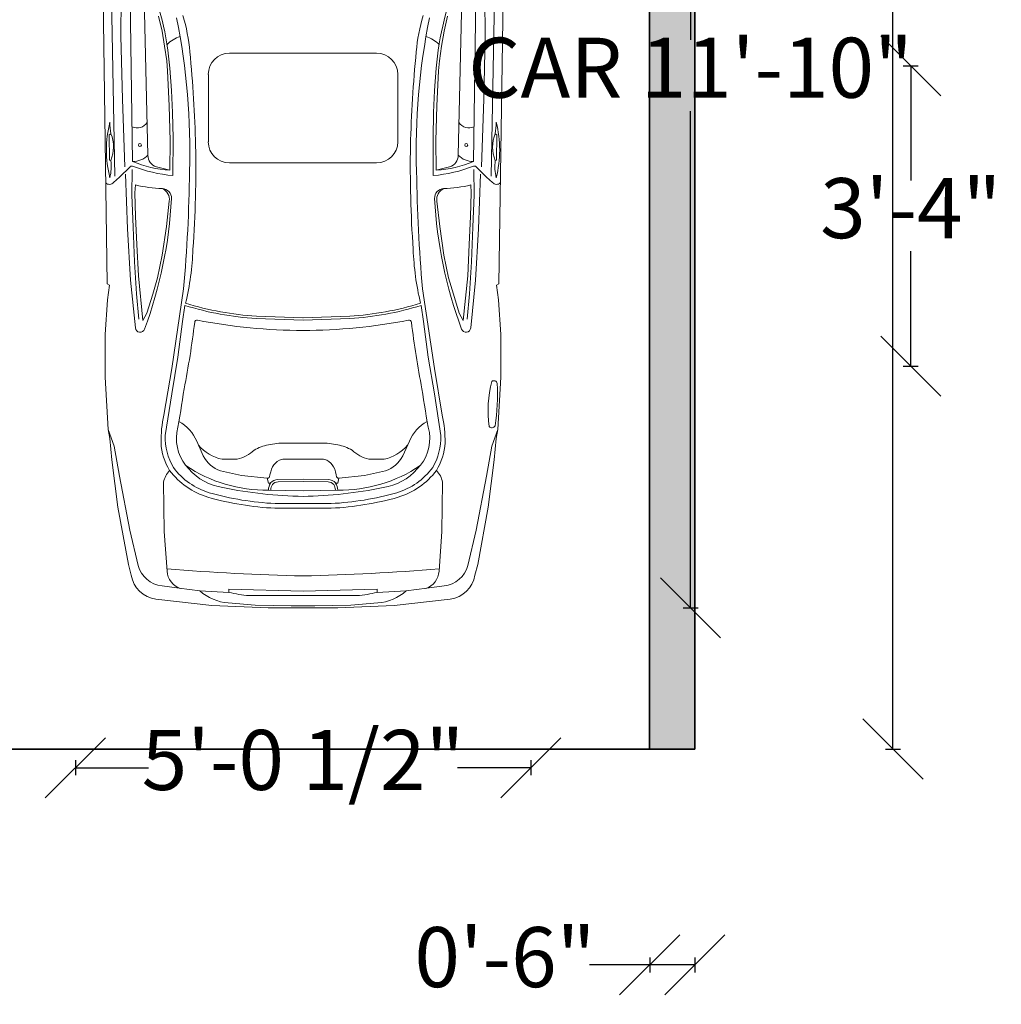
# Model space of a CAD drawing. Units: inches. Extents: x 2247 to 2713, y 588 to 1209.
# Tile 2 of 5: x 2574 to 2705, y 594 to 725. Entities that reach past the tile are written whole.
import ezdxf

# ---------------------------------------------------------------- set-up
doc = ezdxf.new("R2010")
doc.units = ezdxf.units.IN
for name, color, linetype, lineweight in [('0_Equip', 250, 'Continuous', 18), ('A-ANNO-DIMS', 2, 'Continuous', 18), ('A-WALL', 7, 'Continuous', 35), ('A-WALL-PATT', 4, 'Continuous', 13)]:
    doc.layers.add(name, color=color, linetype=linetype, lineweight=lineweight)
doc.styles.get("Standard").update_dxf_attribs({"font": 'arial.ttf'})
doc.dimstyles.new('ISO-25', dxfattribs={"dimtxt": 8, "dimasz": 8, "dimexe": 1, "dimexo": 1, "dimtad": 0, "dimtih": 1, "dimtoh": 1, "dimlunit": 3, "dimtxsty": 'Standard', "dimblk": 'OBLIQUE', "dimcen": 2.5, "dimadec": 0, "dimazin": 0, "dimtfac": 1, "dimtmove": 0, "dimatfit": 3, "dimfxl": 1, "dimfxlon": 1, "dimarcsym": 0})

# ---------------------------------------------------------------- blocks, each defined once
blk = doc.blocks.new('A$C4C7B54D1')
at = {"layer": '0_Equip', "ltscale": 0.1}
for p, q in [((-1.5337, 0.8406), (-1.5355, 0.484)), ((-1.4835, -0.0735), (-1.497, 0.863)), ((0.0322, -0.0735), (0.0457, 0.863)), ((0.0824, 0.8406), (0.0842, 0.484)), ((-1.6171, 0.8152), (-1.5964, -0.6171)), ((-1.5805, 0.8299), (-1.5623, -0.138)), ((-1.4352, 0.792), (-1.4152, -0.045)), ((-0.0162, 0.792), (-0.0361, -0.045)), ((0.1292, 0.8299), (0.111, -0.138)), ((0.1658, 0.8152), (0.145, -0.6171)), ((-1.368, 0.5729), (-1.3527, 0.5066)), ((-0.0834, 0.5729), (-0.0986, 0.5066)), ((-1.5355, 0.484), (-1.5292, 0.2045)), ((-1.3527, 0.5066), (-1.3411, 0.4394)), ((-0.0986, 0.5066), (-0.1102, 0.4394)), ((0.0842, 0.484), (0.0779, 0.2045)), ((-1.3411, 0.4394), (-1.3321, 0.3749)), ((-0.1102, 0.4394), (-0.1192, 0.3749)), ((-0.7257, 0.4085), (-1.0528, 0.4085)), ((-0.7257, 0.4085), (-0.3986, 0.4085)), ((-1.3321, 0.3749), (-1.3286, 0.3301)), ((-0.1192, 0.3749), (-0.1228, 0.3301)), ((-1.3286, 0.3301), (-1.3204, 0.1751)), ((-1.3178, 0.3418), (-1.31, 0.2426)), ((-1.1468, 0.3145), (-1.1468, 0.0145)), ((-0.3045, 0.3145), (-0.3045, 0.0145)), ((-0.1335, 0.3418), (-0.1413, 0.2426)), ((-0.1228, 0.3301), (-0.1309, 0.1751)), ((-1.31, 0.2426), (-1.306, 0.1454)), ((-0.1413, 0.2426), (-0.1454, 0.1454)), ((-1.5292, 0.2045), (-1.5185, -0.0974)), ((0.0779, 0.2045), (0.0672, -0.0974)), ((-1.3204, 0.1751), (-1.3164, 0.0193)), ((-1.306, 0.1454), (-1.3036, 0.0305)), ((-0.1454, 0.1454), (-0.1478, 0.0305)), ((-0.1309, 0.1751), (-0.1349, 0.0193)), ((-1.5798, 0.0505), (-1.5879, 0.0456)), ((-1.5879, 0.0456), (-1.5863, -0.0676)), ((0.1285, 0.0505), (0.1365, 0.0456)), ((0.1365, 0.0456), (0.1349, -0.0676)), ((-1.3164, 0.0193), (-1.3178, -0.1112)), ((-1.3036, 0.0305), (-1.3044, -0.1358)), ((-0.1478, 0.0305), (-0.147, -0.1358)), ((-0.1349, 0.0193), (-0.1335, -0.1112)), ((-1.5863, -0.0676), (-1.5806, -0.0692)), ((-0.7257, -0.0796), (-1.0528, -0.0796)), ((-0.7257, -0.0796), (-0.3986, -0.0796)), ((0.1349, -0.0676), (0.1293, -0.0692)), ((-1.4948, -0.0965), (-1.5413, -0.143)), ((-1.5147, -0.1299), (-1.5058, -0.3725)), ((-1.4857, -0.1082), (-1.4866, -0.2223)), ((-1.3774, -0.0972), (-1.3178, -0.1112)), ((-0.0739, -0.0972), (-0.1335, -0.1112)), ((0.0344, -0.1082), (0.0352, -0.2223)), ((0.0435, -0.0965), (0.0899, -0.143)), ((0.0633, -0.1299), (0.0545, -0.3725)), ((-1.5413, -0.143), (-1.5686, -0.1663)), ((0.0899, -0.143), (0.1172, -0.1663)), ((-1.4713, -0.1773), (-1.4737, -0.2127)), ((-1.4737, -0.2127), (-1.4705, -0.3187)), ((0.0224, -0.2127), (0.0192, -0.3187)), ((0.02, -0.1773), (0.0224, -0.2127)), ((-1.4866, -0.2223), (-1.4809, -0.3653)), ((-1.3211, -0.2496), (-1.3332, -0.3629)), ((-0.1302, -0.2496), (-0.1182, -0.3629)), ((0.0352, -0.2223), (0.0296, -0.3653)), ((-1.4705, -0.3187), (-1.4649, -0.4424)), ((0.0192, -0.3187), (0.0135, -0.4424)), ((-1.5058, -0.3725), (-1.4922, -0.6007)), ((-1.4809, -0.3653), (-1.4745, -0.5203)), ((-1.3332, -0.3629), (-1.3516, -0.4906)), ((-0.1182, -0.3629), (-0.0997, -0.4906)), ((0.0296, -0.3653), (0.0232, -0.5203)), ((0.0545, -0.3725), (0.0408, -0.6007)), ((-1.4649, -0.4424), (-1.4576, -0.5822)), ((0.0135, -0.4424), (0.0063, -0.5822)), ((-1.4745, -0.5203), (-1.4665, -0.6617)), ((-1.3516, -0.4906), (-1.3725, -0.5902)), ((-0.0997, -0.4906), (-0.0788, -0.5902)), ((0.0232, -0.5203), (0.0151, -0.6617)), ((-1.4922, -0.6007), (-1.4712, -0.814)), ((-1.4576, -0.5822), (-1.4384, -0.7806)), ((-1.3725, -0.5902), (-1.3942, -0.6641)), ((-0.0788, -0.5902), (-0.0571, -0.6641)), ((0.0063, -0.5822), (-0.013, -0.7806)), ((0.0408, -0.6007), (0.0198, -0.814)), ((-1.5964, -0.6171), (-1.5863, -0.6228)), ((-1.5863, -0.6228), (-1.5949, -0.6885)), ((-1.3094, -0.9936), (-1.2569, -0.6398)), ((-0.1419, -0.9936), (-0.1944, -0.6398)), ((0.145, -0.6171), (0.1349, -0.6228)), ((0.1349, -0.6228), (0.1436, -0.6885)), ((-1.5949, -0.6885), (-1.605, -0.843)), ((-1.4665, -0.6617), (-1.4552, -0.7742)), ((-1.3942, -0.6641), (-1.4199, -0.7485)), ((-0.0571, -0.6641), (-0.0314, -0.7485)), ((0.0151, -0.6617), (0.0039, -0.7742)), ((0.1436, -0.6885), (0.1537, -0.843)), ((-1.2616, -0.7846), (-1.2511, -0.7134)), ((-0.1898, -0.7846), (-0.2003, -0.7134)), ((-1.4199, -0.7485), (-1.4384, -0.7806)), ((-1.2826, -0.9445), (-1.2616, -0.7846)), ((-0.9336, -0.7717), (-0.7257, -0.7787)), ((-0.9331, -0.7613), (-0.7253, -0.7683)), ((-0.5182, -0.7613), (-0.726, -0.7683)), ((-0.5177, -0.7717), (-0.7257, -0.7787)), ((-0.1688, -0.9445), (-0.1898, -0.7846)), ((-0.0314, -0.7485), (-0.013, -0.7806)), ((-1.605, -0.843), (-1.605, -1.0322)), ((0.1537, -0.843), (0.1537, -1.0322)), ((-1.3094, -1.1068), (-1.2826, -0.9445)), ((-0.1419, -1.1068), (-0.1688, -0.9445)), ((-1.3444, -1.2014), (-1.3094, -0.9936)), ((-0.1069, -1.2014), (-0.1419, -0.9936)), ((-1.605, -1.0322), (-1.592, -1.2661)), ((0.1537, -1.0322), (0.1407, -1.2661)), ((-1.3386, -1.2925), (-1.3094, -1.1068)), ((-0.1127, -1.2925), (-0.1419, -1.1068)), ((-1.565, -1.3405), (-1.592, -1.2661)), ((-1.592, -1.2661), (-1.5848, -1.3051)), ((0.1137, -1.3405), (0.1407, -1.2661)), ((0.1407, -1.2661), (0.1335, -1.3051)), ((-1.5848, -1.3051), (-1.5762, -1.4004)), ((0.1335, -1.3051), (0.1248, -1.4004)), ((-1.5417, -1.4736), (-1.565, -1.3405)), ((-1.1985, -1.3182), (-1.1694, -1.3835)), ((-0.88, -1.3337), (-0.8328, -1.3271)), ((-0.8328, -1.3271), (-0.7257, -1.3271)), ((-0.6185, -1.3271), (-0.7257, -1.3271)), ((-0.5713, -1.3337), (-0.6185, -1.3271)), ((-0.2528, -1.3182), (-0.282, -1.3835)), ((0.0904, -1.4736), (0.1137, -1.3405)), ((-1.5762, -1.4004), (-1.5486, -1.6107)), ((-1.0858, -1.3979), (-1.0181, -1.3979)), ((-0.8163, -1.3979), (-0.8309, -1.402)), ((-0.7257, -1.3974), (-0.8163, -1.3979)), ((-0.7257, -1.3974), (-0.635, -1.3979)), ((-0.635, -1.3979), (-0.6204, -1.402)), ((-0.3655, -1.3979), (-0.4333, -1.3979)), ((0.1248, -1.4004), (0.0973, -1.6107)), ((-0.8664, -1.4423), (-0.8696, -1.4545)), ((-0.861, -1.4312), (-0.8664, -1.4423)), ((-0.8558, -1.4236), (-0.861, -1.4312)), ((-0.8488, -1.4158), (-0.8558, -1.4236)), ((-0.8409, -1.4088), (-0.8488, -1.4158)), ((-0.8309, -1.402), (-0.8409, -1.4088)), ((-0.6204, -1.402), (-0.6104, -1.4088)), ((-0.6104, -1.4088), (-0.6025, -1.4158)), ((-0.6025, -1.4158), (-0.5955, -1.4236)), ((-0.5955, -1.4236), (-0.5904, -1.4312)), ((-0.5904, -1.4312), (-0.585, -1.4423)), ((-0.585, -1.4423), (-0.5817, -1.4545)), ((-1.4962, -1.7129), (-1.5417, -1.4736)), ((-1.0923, -1.4501), (-0.9989, -1.4699)), ((-0.9989, -1.4699), (-0.8846, -1.4828)), ((-0.8807, -1.4821), (-0.8846, -1.4828)), ((-0.8846, -1.4828), (-0.8799, -1.5038)), ((-0.8769, -1.4791), (-0.8807, -1.4821)), ((-0.8745, -1.477), (-0.8769, -1.4791)), ((-0.8731, -1.467), (-0.8745, -1.477)), ((-0.8696, -1.4545), (-0.8731, -1.467)), ((-0.7257, -1.4865), (-0.8374, -1.4884)), ((-0.7257, -1.4865), (-0.6139, -1.4884)), ((-0.5817, -1.4545), (-0.5782, -1.467)), ((-0.5782, -1.467), (-0.5768, -1.477)), ((-0.5768, -1.477), (-0.5744, -1.4791)), ((-0.5744, -1.4791), (-0.5706, -1.4821)), ((-0.5668, -1.4828), (-0.5714, -1.5038)), ((-0.5706, -1.4821), (-0.5668, -1.4828)), ((-0.4524, -1.4699), (-0.5668, -1.4828)), ((-0.359, -1.4501), (-0.4524, -1.4699)), ((0.0448, -1.7129), (0.0904, -1.4736)), ((-1.3456, -1.5004), (-1.3433, -1.7188)), ((-0.8799, -1.5038), (-0.8706, -1.5038)), ((-0.7257, -1.4969), (-0.837, -1.4988)), ((-0.7257, -1.4969), (-0.6143, -1.4988)), ((-0.5714, -1.5038), (-0.5808, -1.5038)), ((-0.1057, -1.5004), (-0.1081, -1.7188)), ((-0.8799, -1.5352), (-0.7257, -1.5393)), ((-0.5714, -1.5352), (-0.7257, -1.5393)), ((-1.5486, -1.6107), (-1.5024, -1.8663)), ((-0.8507, -1.616), (-0.7257, -1.616)), ((-0.8502, -1.5951), (-0.7257, -1.5951)), ((-0.6011, -1.5951), (-0.7257, -1.5951)), ((-0.6006, -1.616), (-0.7257, -1.616)), ((0.0973, -1.6107), (0.0511, -1.8663)), ((-1.4584, -1.8701), (-1.4962, -1.7129)), ((-1.3433, -1.7188), (-1.3304, -1.8962)), ((-0.1081, -1.7188), (-0.1209, -1.8962)), ((0.0071, -1.8701), (0.0448, -1.7129)), ((-1.5024, -1.8663), (-1.4894, -1.914)), ((0.0511, -1.8663), (0.0381, -1.914)), ((-1.2767, -1.9721), (-1.3526, -1.9616)), ((-0.1746, -1.9721), (-0.0987, -1.9616)), ((-1.1845, -1.9838), (-1.2767, -1.9721)), ((-1.055, -1.9908), (-1.1845, -1.9838)), ((-1.055, -1.9768), (-1.055, -1.9908)), ((-0.7257, -1.985), (-1.055, -1.9768)), ((-0.9663, -2.0048), (-0.7257, -2.0048)), ((-0.7257, -1.985), (-0.3964, -1.9768)), ((-0.4851, -2.0048), (-0.7257, -2.0048)), ((-0.3964, -1.9768), (-0.3964, -1.9908)), ((-0.3964, -1.9908), (-0.2668, -1.9838)), ((-0.2668, -1.9838), (-0.1746, -1.9721)), ((-1.3797, -2.0208), (-1.1314, -2.0483)), ((-1.1314, -2.0483), (-0.8803, -2.0598)), ((-1.0585, -2.0375), (-0.9383, -2.0469)), ((-0.9383, -2.0469), (-0.7784, -2.0504)), ((-0.7784, -2.0504), (-0.7257, -2.0504)), ((-0.673, -2.0504), (-0.7257, -2.0504)), ((-0.5131, -2.0469), (-0.673, -2.0504)), ((-0.3199, -2.0483), (-0.5711, -2.0598)), ((-0.3929, -2.0375), (-0.5131, -2.0469)), ((-0.0716, -2.0208), (-0.3199, -2.0483)), ((-0.8803, -2.0598), (-0.7257, -2.0598)), ((-0.5711, -2.0598), (-0.7257, -2.0598))]:
    blk.add_line(p, q, dxfattribs=at)
for centre in [(-1.4513, 0), (0, 0)]:
    blk.add_circle(centre, 0.00662, dxfattribs=at)
for centre, radius, start, end in [((-6.6059, -0.8606), 5.4408, 15.0904, 20.5451), ((5.1546, -0.8606), 5.4408, 159.4549, 164.9096), ((-2.0025, 0.3511), 0.7759, 4.7259, 16.8296), ((0.5512, 0.3511), 0.7759, 163.1704, 175.2741), ((-2.6334, 0.2371), 1.3197, 4.5498, 13.9797), ((-4.2099, -0.0242), 2.9809, 358.1905, 11.4064), ((2.7585, -0.0242), 2.9809, 168.5936, 181.8095), ((1.1821, 0.2371), 1.3197, 166.0203, 175.4502), ((-1.2324, 0.3484), 0.1397, 106.6168, 134.6647), ((-0.2189, 0.3484), 0.1397, 45.3353, 73.3832), ((-6.5594, -0.126), 5.3575, 1.3159, 5.7952), ((-1.0528, 0.3145), 0.0941, 90, 180), ((-0.3986, 0.3145), 0.0941, 0, 90), ((5.1081, -0.126), 5.3575, 174.2048, 178.6841), ((-1.0944, -0.0222), 0.5055, 165.8807, 194.1193), ((-1.3066, 0.102), 0.2781, 180.1936, 190.6834), ((-1.4634, 0.1296), 0.0534, 245.2796, 326.9469), ((0.0121, 0.1296), 0.0534, 213.0531, 294.7204), ((-0.1448, 0.102), 0.2781, 349.3166, 359.8064), ((-0.3569, -0.0222), 0.5055, 345.8807, 14.1193), ((-1.7275, -0.0084), 0.159, 337.4976, 21.7335), ((0.2762, -0.0084), 0.159, 158.2665, 202.5024), ((-1.0528, 0.0145), 0.0941, 180, 270), ((-0.3986, 0.0145), 0.0941, 270, 0), ((-6.573, -0.0941), 5.3705, 356.0501, 0.9723), ((5.1217, -0.0941), 5.3705, 179.0277, 183.9499), ((-1.7817, -0.0969), 0.2029, 346.1346, 7.8419), ((-1.4831, 0.0214), 0.095, 269.7172, 315.6185), ((-1.2968, 0.3651), 0.4767, 246.9385, 267.4714), ((-1.3634, -0.0473), 0.0519, 177.4537, 254.2676), ((-0.1545, 0.3651), 0.4767, 272.5286, 293.0615), ((-0.0879, -0.0473), 0.0519, 285.7324, 2.5463), ((0.0317, 0.0214), 0.095, 224.3815, 270.2828), ((0.3303, -0.0969), 0.2029, 172.1581, 193.8654), ((-1.4874, -0.1039), 0.0105, 68.8598, 135.0096), ((-1.2476, 0.5164), 0.6547, 248.8598, 265.0222), ((-8.0298, -0.0355), 6.7998, 354.90123, 359.30214), ((6.5785, -0.0355), 6.7998, 180.69786, 185.09877), ((-0.2038, 0.5164), 0.6547, 274.9778, 291.1402), ((0.0361, -0.1039), 0.0105, 44.9904, 111.1402), ((-1.5869, -0.1514), 0.0236, 227.2909, 320.7388), ((0.1355, -0.1514), 0.0236, 219.2612, 312.7091), ((-1.3362, 0.3542), 0.5484, 255.7347, 268.4072), ((-1.3699, -0.2402), 0.0497, 349.0381, 68.1064), ((-1.3526, -0.2358), 0.0418, 357.143, 88.4072), ((-0.0988, -0.2358), 0.0418, 91.5928, 182.857), ((-0.0814, -0.2402), 0.0497, 111.8936, 190.9619), ((-0.1152, 0.3542), 0.5484, 271.5928, 284.2653), ((-3.2483, -0.1412), 1.9399, 339.54, 357.143), ((1.797, -0.1412), 1.9399, 182.857, 200.46), ((-2.454, -0.4173), 1.2396, 346.6558, 357.8401), ((1.0027, -0.4173), 1.2396, 182.1599, 193.3442), ((-0.8588, 0.5276), 1.3014, 252.4566, 266.7043), ((-0.8588, 0.5276), 1.291, 252.4566, 266.6988), ((-0.5926, 0.5276), 1.291, 273.3012, 287.5434), ((-0.5926, 0.5276), 1.3014, 273.2957, 287.5434), ((-1.1971, -0.7899), 0.0105, 79.1189, 173.1671), ((-0.7142, 1.7227), 2.5481, 259.1189, 269.7413), ((-0.7372, 1.7227), 2.5481, 270.2587, 280.8811), ((-0.2542, -0.7899), 0.0105, 6.8329, 100.8811), ((-1.4504, -0.812), 0.0209, 185.6259, 339.54), ((-5.088, -0.3237), 3.9082, 348.7726, 353.1671), ((3.6366, -0.3237), 3.9082, 186.8329, 191.2274), ((-0.001, -0.812), 0.0209, 200.46, 354.3741), ((0.1224, -1.0639), 0.0155, 11.61, 127.0083), ((-4.7286, -0.6026), 3.5073, 348.8701, 352.1003), ((3.2772, -0.6026), 3.5073, 187.8997, 191.1299), ((0.625, -1.1812), 0.5281, 165.7822, 187.813), ((-0.7003, -1.1122), 0.8395, 350.5693, 3.5107), ((-0.8187, -1.3185), 0.5386, 167.4447, 180.7102), ((-0.6326, -1.3185), 0.5386, 359.2898, 12.5553), ((-1.3591, -1.3822), 0.1728, 21.7432, 61.9432), ((-0.0922, -1.3822), 0.1728, 118.0568, 158.2568), ((0.1138, -1.243), 0.0156, 219.7819, 334.4738), ((-1.0611, -1.2979), 0.2775, 178.8811, 209.7062), ((-1.0952, -1.3051), 0.1937, 172.4314, 224.4267), ((-0.3561, -1.3051), 0.1937, 315.5733, 7.5686), ((-0.3902, -1.2979), 0.2775, 330.2938, 1.1189), ((-1.0944, -1.3104), 0.2633, 183.2136, 211.504), ((-1.0482, -1.2146), 0.1871, 220.4031, 258.3959), ((-1.0495, -1.2507), 0.1505, 282.0448, 314.7653), ((-0.8301, -1.5634), 0.235, 102.268, 118.8572), ((-0.6213, -1.5634), 0.235, 61.1428, 77.732), ((-0.4019, -1.2507), 0.1505, 225.2347, 257.9552), ((-0.4032, -1.2146), 0.1871, 281.6041, 319.5969), ((-0.3569, -1.3104), 0.2633, 328.496, 356.7864), ((-1.0421, -1.3141), 0.145, 208.6187, 249.7318), ((-0.4092, -1.3141), 0.145, 290.2682, 331.3813), ((-1.052, -1.2472), 0.313, 216.9484, 253.2054), ((-0.8912, -0.9022), 0.6331, 235.8724, 271.0227), ((-1.0459, -1.2776), 0.2487, 221.0065, 261.6946), ((-0.5601, -0.9022), 0.6331, 268.9773, 304.1276), ((-0.4054, -1.2776), 0.2487, 278.3054, 318.9935), ((-0.3993, -1.2472), 0.313, 286.7946, 323.0516), ((-1.2501, -1.516), 0.0967, 135.2951, 170.7274), ((-1.052, -1.2472), 0.3339, 216.9484, 253.2314), ((-0.8344, -1.538), 0.0498, 93.4455, 136.5439), ((-0.6169, -1.538), 0.0498, 43.4561, 86.5545), ((-0.3993, -1.2472), 0.3339, 286.7686, 323.0516), ((-0.2012, -1.516), 0.0967, 9.2726, 44.7049), ((-0.7003, 0.2815), 1.8451, 258.0669, 269.2129), ((-0.8066, -1.54), 0.0735, 150.5285, 176.2825), ((-0.8066, -1.54), 0.063, 151.7195, 175.9212), ((-0.8344, -1.538), 0.0393, 93.7549, 134.7116), ((-0.751, 0.2815), 1.8451, 270.7871, 281.9331), ((-0.6169, -1.538), 0.0393, 45.2884, 86.2451), ((-0.6447, -1.54), 0.063, 4.0788, 28.2805), ((-0.6447, -1.54), 0.0735, 3.7175, 29.4715), ((-0.7884, -0.3101), 1.3074, 254.0198, 267.2681), ((-0.7884, -0.3101), 1.2865, 254.0263, 267.246), ((-0.6629, -0.3101), 1.2865, 272.754, 285.9737), ((-0.6629, -0.3101), 1.3074, 272.7319, 285.9802), ((-1.3393, -1.8393), 0.123, 194.4986, 263.7836), ((-0.1121, -1.8393), 0.123, 276.2164, 345.5014), ((-1.3628, -1.8937), 0.1282, 189.093, 262.4153), ((-0.5134, 7.9307), 9.8503, 265.23745, 268.76503), ((-1.2452, -1.8915), 0.0853, 183.2055, 252.6405), ((-0.938, 7.9307), 9.8503, 271.23497, 274.76255), ((-0.2061, -1.8915), 0.0853, 287.3595, 356.7945), ((-0.0885, -1.8937), 0.1282, 277.5847, 350.907), ((-1.0413, -1.8225), 0.2157, 228.406, 265.4391), ((-0.896, -1.272), 0.7362, 257.5275, 264.5209), ((-0.5554, -1.272), 0.7362, 275.4791, 282.4725), ((-0.41, -1.8225), 0.2157, 274.5609, 311.594)]:
    blk.add_arc(centre, radius, start, end, dxfattribs=at)
blk = doc.blocks.new('_Oblique')
at = {"color": 0, "linetype": 'ByBlock', "lineweight": -2}
blk.add_line((-0.5, -0.5), (0.5, 0.5), dxfattribs=at)
blk = doc.blocks.new('*D12')
at = {"layer": 'A-ANNO-DIMS', "color": 0, "lineweight": -2, "transparency": 16777216}
for p, q in [((2689.46, 1168.28), (2691.46, 1168.28)), ((2690.46, 1168.28), (2690.46, 902.97)), ((2690.46, 628.28), (2690.46, 893.59)), ((2689.46, 628.28), (2691.46, 628.28))]:
    blk.add_line(p, q, dxfattribs=at)
at = {"layer": 'Defpoints', "color": 0, "transparency": 16777216}
for p in [(2664.08, 1168.28), (2664.08, 628.28), (2690.46, 628.28)]:
    blk.add_point(p, dxfattribs=at)
at = {"layer": 'A-ANNO-DIMS', "color": 0, "lineweight": -2, "transparency": 16777216, "xscale": 8, "yscale": 8, "zscale": 8}
for p, rotation in [((2690.46, 1168.28), 90), ((2690.46, 628.28), 270)]:
    blk.add_blockref('_Oblique', p, dxfattribs=dict(at, rotation=rotation))
at = {"layer": 'A-ANNO-DIMS', "color": 0, "transparency": 16777216, "insert": (2690.46, 898.28), "char_height": 8, "attachment_point": 5}
blk.add_mtext("45'", dxfattribs=at)
blk = doc.blocks.new('*D23')
at = {"layer": 'A-ANNO-DIMS', "color": 0, "lineweight": -2, "transparency": 16777216}
for p, q in [((2662.52, 788.89), (2664.52, 788.89)), ((2663.52, 788.89), (2663.52, 722.74)), ((2663.52, 647.07), (2663.52, 713.22)), ((2662.52, 647.07), (2664.52, 647.07))]:
    blk.add_line(p, q, dxfattribs=at)
at = {"layer": 'Defpoints', "color": 0, "transparency": 16777216}
for p in [(2642.25, 788.89), (2663.52, 788.89), (2642.25, 647.07)]:
    blk.add_point(p, dxfattribs=at)
at = {"layer": 'A-ANNO-DIMS', "color": 0, "lineweight": -2, "transparency": 16777216, "xscale": 8, "yscale": 8, "zscale": 8}
for p, rotation in [((2663.52, 788.89), 90), ((2663.52, 647.07), 270)]:
    blk.add_blockref('_Oblique', p, dxfattribs=dict(at, rotation=rotation))
at = {"layer": 'A-ANNO-DIMS', "color": 0, "transparency": 16777216, "insert": (2663.52, 717.98), "char_height": 8, "attachment_point": 5}
blk.add_mtext('CAR 11\'-10"', dxfattribs=at)
blk = doc.blocks.new('*D24')
at = {"layer": 'A-ANNO-DIMS', "color": 0, "lineweight": -2, "transparency": 16777216}
for p, q in [((2581.64, 626.79), (2581.64, 624.79)), ((2581.64, 625.79), (2591.36, 625.79)), ((2642.25, 625.79), (2632.52, 625.79)), ((2642.25, 626.79), (2642.25, 624.79))]:
    blk.add_line(p, q, dxfattribs=at)
at = {"layer": 'Defpoints', "color": 0, "transparency": 16777216}
for p in [(2581.64, 647.07), (2642.25, 647.07), (2642.25, 625.79)]:
    blk.add_point(p, dxfattribs=at)
at = {"layer": 'A-ANNO-DIMS', "color": 0, "lineweight": -2, "transparency": 16777216, "xscale": 8, "yscale": 8, "zscale": 8, "rotation": 180}
blk.add_blockref('_Oblique', (2581.64, 625.79), dxfattribs=at)
at = {"layer": 'A-ANNO-DIMS', "color": 0, "lineweight": -2, "transparency": 16777216, "xscale": 8, "yscale": 8, "zscale": 8}
blk.add_blockref('_Oblique', (2642.25, 625.79), dxfattribs=at)
at = {"layer": 'A-ANNO-DIMS', "color": 0, "transparency": 16777216, "insert": (2611.94, 625.79), "char_height": 8, "attachment_point": 5}
blk.add_mtext('5\'-0 1/2"', dxfattribs=at)
blk = doc.blocks.new('*D25')
at = {"layer": 'A-ANNO-DIMS', "color": 0, "lineweight": -2, "transparency": 16777216}
for p, q in [((2691.83, 719.28), (2693.83, 719.28)), ((2692.83, 719.28), (2692.83, 703.99)), ((2692.83, 679.28), (2692.83, 694.57)), ((2691.83, 679.28), (2693.83, 679.28))]:
    blk.add_line(p, q, dxfattribs=at)
at = {"layer": 'Defpoints', "color": 0, "transparency": 16777216}
for p in [(2520.08, 719.28), (2692.83, 719.28), (2520.08, 679.28)]:
    blk.add_point(p, dxfattribs=at)
at = {"layer": 'A-ANNO-DIMS', "color": 0, "lineweight": -2, "transparency": 16777216, "xscale": 8, "yscale": 8, "zscale": 8}
for p, rotation in [((2692.83, 719.28), 90), ((2692.83, 679.28), 270)]:
    blk.add_blockref('_Oblique', p, dxfattribs=dict(at, rotation=rotation))
at = {"layer": 'A-ANNO-DIMS', "color": 0, "transparency": 16777216, "insert": (2692.83, 699.28), "char_height": 8, "attachment_point": 5}
blk.add_mtext('3\'-4"', dxfattribs=at)
blk = doc.blocks.new('*D28')
at = {"layer": 'A-ANNO-DIMS', "color": 0, "lineweight": -2, "transparency": 16777216}
for p, q in [((2658.08, 599.53), (2650.08, 599.53)), ((2658.08, 600.53), (2658.08, 598.53)), ((2664.08, 599.53), (2658.08, 599.53)), ((2664.08, 600.53), (2664.08, 598.53))]:
    blk.add_line(p, q, dxfattribs=at)
at = {"layer": 'Defpoints', "color": 0, "transparency": 16777216}
for p in [(2658.08, 628.28), (2664.08, 628.28), (2658.08, 599.53)]:
    blk.add_point(p, dxfattribs=at)
at = {"layer": 'A-ANNO-DIMS', "color": 0, "lineweight": -2, "transparency": 16777216, "xscale": 8, "yscale": 8, "zscale": 8, "rotation": 180}
blk.add_blockref('_Oblique', (2658.08, 599.53), dxfattribs=at)
at = {"layer": 'A-ANNO-DIMS', "color": 0, "lineweight": -2, "transparency": 16777216, "xscale": 8, "yscale": 8, "zscale": 8}
blk.add_blockref('_Oblique', (2664.08, 599.53), dxfattribs=at)
at = {"layer": 'A-ANNO-DIMS', "color": 0, "transparency": 16777216, "insert": (2638.82, 599.53), "char_height": 8, "attachment_point": 5}
blk.add_mtext('0\'-6"', dxfattribs=at)

msp = doc.modelspace()

# ---------------------------------------------------------------- hatches: boundary and pattern name
at = {"layer": 'A-WALL-PATT'}
h = msp.add_hatch(color=256, dxfattribs=at)
h.dxf.hatch_style = 1
h.paths.add_polyline_path([(2604.041, 1168.28), (2423.716, 1168.28), (2423.716, 1162.28), (2442.076, 1162.28), (2442.076, 1114.28), (2439.021, 1114.28), (2439.021, 1108.28), (2456.056, 1108.28), (2456.056, 1114.28), (2448.076, 1114.28), (2448.076, 1162.28), (2580.076, 1162.28), (2580.076, 1114.28), (2560.507, 1114.28), (2560.507, 1108.28), (2619.195, 1108.28), (2619.195, 1114.28), (2586.076, 1114.28), (2586.076, 1162.28), (2604.041, 1162.28)])
h.paths.add_polyline_path([(2380.833, 1168.28), (2364.076, 1168.28), (2364.076, 1094.128), (2370.076, 1094.128), (2370.076, 1108.28), (2407.021, 1108.28), (2407.021, 1114.28), (2370.076, 1114.28), (2370.076, 1162.28), (2380.833, 1162.28)])
h.paths.add_polyline_path([(2664.076, 1168.28), (2639.393, 1168.28), (2639.393, 1162.28), (2658.076, 1162.28), (2658.076, 1114.28), (2651.195, 1114.28), (2651.195, 1108.28), (2658.076, 1108.28), (2658.076, 1094.128), (2664.076, 1094.128)])
h.paths.add_polyline_path([(2524.66, 1114.28), (2487.371, 1114.28), (2487.371, 1108.28), (2511.076, 1108.28), (2511.076, 940.28), (2508.076, 940.28), (2508.076, 934.28), (2520.076, 934.28), (2520.076, 940.28), (2517.076, 940.28), (2517.076, 1108.28), (2524.66, 1108.28)])
h.paths.add_polyline_path([(2370.076, 1054.172), (2364.076, 1054.172), (2364.076, 990.686), (2370.076, 990.686)])
h.paths.add_polyline_path([(2370.076, 934.28), (2472.076, 934.28), (2472.076, 940.28), (2370.076, 940.28), (2370.076, 950.99), (2364.076, 950.99), (2364.076, 902.687), (2370.076, 902.687)])
h.paths.add_polyline_path([(2664.076, 950.99), (2658.076, 950.99), (2658.076, 940.28), (2556.076, 940.28), (2556.076, 934.28), (2658.076, 934.28), (2658.076, 913.24), (2664.076, 913.24)])
h.paths.add_polyline_path([(2664.076, 1054.172), (2658.076, 1054.172), (2658.076, 990.686), (2664.076, 990.686)])
h.paths.add_polyline_path([(2664.076, 861.585), (2658.076, 861.585), (2658.076, 814.28), (2626.201, 814.28), (2626.201, 808.28), (2658.076, 808.28), (2658.076, 628.28), (2664.076, 628.28)])
h.paths.add_polyline_path([(2562.076, 871.28), (2556.076, 871.28), (2556.076, 808.28), (2584.934, 808.28), (2584.934, 814.28), (2562.076, 814.28)])
h.paths.add_polyline_path([(2475.722, 808.28), (2370.076, 808.28), (2370.076, 776.746), (2364.076, 776.746), (2364.076, 846.663), (2370.076, 846.663), (2370.076, 814.28), (2475.722, 814.28)])
h.paths.add_polyline_path([(2370.076, 709.673), (2364.076, 709.673), (2364.076, 628.28), (2520.076, 628.28), (2520.076, 634.28), (2370.076, 634.28)])
h.paths.add_polyline_path([(2410.479, 679.28), (2370.076, 679.28), (2370.076, 673.28), (2410.479, 673.28)], flags=17)
h.paths.add_polyline_path([(2520.076, 679.28), (2514.076, 679.28), (2474.076, 679.28), (2457.582, 679.28), (2457.582, 673.28), (2520.076, 673.28)], flags=17)
h.paths.add_polyline_path([(2520.076, 814.28), (2511.722, 814.28), (2511.722, 808.28), (2514.076, 808.28), (2514.076, 719.28), (2520.076, 719.28)])

# ---------------------------------------------------------------- linework, layer by layer
at = {"layer": 'A-WALL'}
for p, q in [((2664.076, 628.28), (2664.076, 1168.28)), ((2658.076, 628.28), (2658.076, 808.28)), ((2364.076, 628.28), (2664.076, 628.28))]:
    msp.add_line(p, q, dxfattribs=at)

# ---------------------------------------------------------------- block references
at = {"layer": '0_Equip', "xscale": 29.93372244382068, "yscale": 29.93372244382068, "zscale": 29.93372244382068}
msp.add_blockref('A$C4C7B54D1', (2633.665, 708.724), dxfattribs=at)

# ---------------------------------------------------------------- dimensions: what is measured, and where the dimension line sits
at = {"layer": 'A-ANNO-DIMS'}
for base, p1, p2, override, picture, middle in [((2690.46, 628.28), (2664.076, 1168.28), (2664.076, 628.28), {"dimclrd": 0, "dimclre": 0, "dimclrt": 0}, '*D12', (2690.46, 898.28)), ((2692.826, 719.28), (2520.076, 679.28), (2520.076, 719.28), {"dimdec": 1, "dimlfac": 1, "dimrnd": 0, "dimzin": 1, "dimdsep": 46, "dimlunit": 4, "dimfrac": 2}, '*D25', (2692.826, 699.28))]:
    dim = msp.add_linear_dim(base=base, p1=p1, p2=p2, angle=90, dimstyle='ISO-25', override=override, dxfattribs=at)
    dim.commit()
    dim.dimension.update_dxf_attribs({"geometry": picture, "text_midpoint": middle})
dim = msp.add_linear_dim(base=(2663.521, 788.887), p1=(2642.248, 647.066), p2=(2642.248, 788.887), angle=90, text='CAR <>', dimstyle='ISO-25', override={"dimdec": 1, "dimlfac": 1, "dimrnd": 0, "dimzin": 1, "dimdsep": 46, "dimlunit": 4, "dimfrac": 2}, dxfattribs=at)
dim.commit()
dim.dimension.update_dxf_attribs({"geometry": '*D23', "text_midpoint": (2663.521, 717.977)})
for base, p1, p2, picture, middle in [((2642.248, 625.793), (2581.638, 647.066), (2642.248, 647.066), '*D24', (2611.943, 625.793)), ((2658.076, 599.53), (2664.076, 628.28), (2658.076, 628.28), '*D28', (2638.818, 599.53))]:
    dim = msp.add_linear_dim(base=base, p1=p1, p2=p2, dimstyle='ISO-25', override={"dimdec": 1, "dimlfac": 1, "dimrnd": 0, "dimzin": 1, "dimdsep": 46, "dimlunit": 4, "dimfrac": 2}, dxfattribs=at)
    dim.commit()
    dim.dimension.update_dxf_attribs({"geometry": picture, "text_midpoint": middle})

doc.saveas('drawing.dxf')
